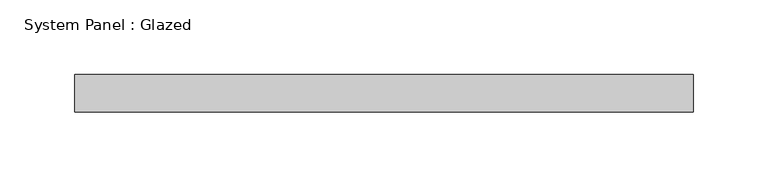
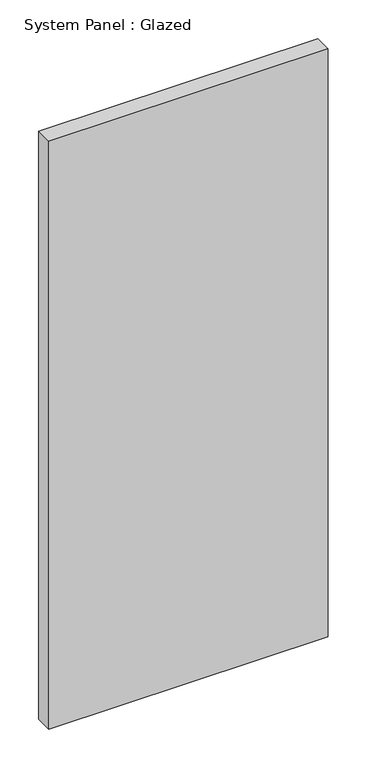
"""IFC4 building model written with IfcOpenShell, lengths in millimetres: plate geometry, System Panel : Glazed."""

from ifc_helpers import new_model, si_unit, origin, origin_with_axes, place, context, project, spatial, polyline, outline, extrude, source, transform, mapped, element, save


def system_panel_glazed_0f72cd4c(model_context):
    return source(origin(), model_context, "Body", "SweptSolid", [
        extrude(outline(polyline([(207.5694345, 19.05), (-207.5694345, 19.05), (-207.5694345, 44.45), (207.5694345, 44.45), (207.5694345, 19.05)])), origin_with_axes(), (0.0, 0.0, 1.0), 923.1640555),
    ])


if __name__ == "__main__":
    model = new_model("IFC4")
    model_context = context("Model", 3, world=origin())
    ifc_project = project(units=[si_unit("LENGTHUNIT", "METRE", prefix="MILLI")], contexts=[model_context])
    site = spatial("IfcSite", under=ifc_project)
    building = spatial("IfcBuilding", under=site)
    placement = place(None, origin())
    system_panel_glazed_shape = system_panel_glazed_0f72cd4c(model_context)
    element("IfcPlate", 1, ObjectType="System Panel : Glazed", at=placement, inside=building, context=model_context, shape_type="MappedRepresentation", body=[
        mapped(system_panel_glazed_shape, transform((0.0, 0.0, 0.0), x_axis=(1.0, 0.0, 0.0), y_axis=(0.0, 1.0, 0.0), z_axis=(0.0, 0.0, 1.0))),
    ])
    save(model, "model.ifc")

# Revit data of these elements
# Type "System Panel : Glazed"
#   Construction Type Id = "GSP4R"
#   Analytic Construction = "1/8 in Pilkington single glazing"
#   Visual Light Transmittance = 0.9
#   Solar Heat Gain Coefficient = 0.86
#   Heat Transfer Coefficient (U) = 1.18115 BTU/(h·ft²·°F)
# Element 1 (IfcPlate, "System Panel : Glazed")
#   Materials on its faces: "Glass"
# Materials
#   "Glass": class "Glass", colour RGB 0 128 192, transparency 0.75, Description = "Soda Lime Glass", Cost = 0
